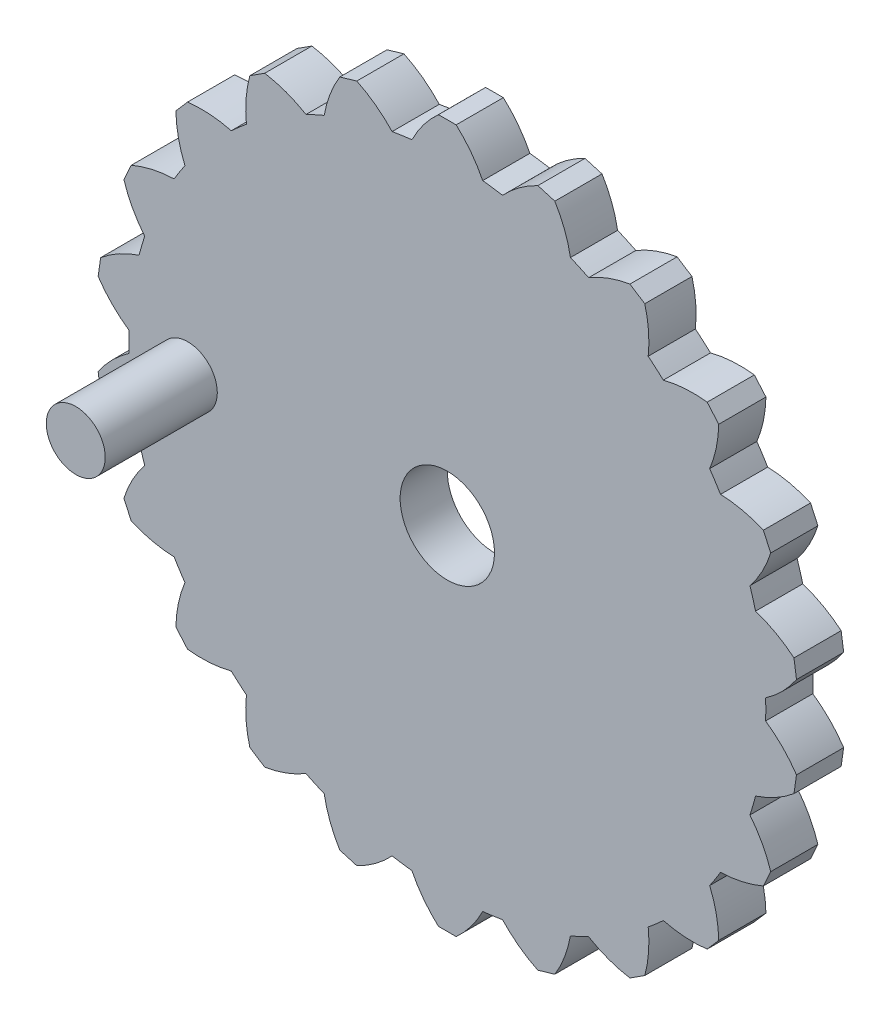
from build123d import *

# Parameters (mm, degrees)
GEAR_PROFILE_SKETCH_R = 4
GEAR_BODY_22T_DEPTH   = 4
SKETCH1_3_R           = 2.5
HUB_BOSS_DEPTH        = 9.5


with BuildPart() as part:
    # Gear Profile Sketch → Gear Body 22T (new body)
    with BuildSketch(Plane.XY):
        with BuildLine():
            Line((-0.75, 29.8), (0.75, 29.8))
            ThreePointArc((0.75, 29.8), (2.014333197, 28.422063485), (3, 26.83281573))
            ThreePointArc((3, 26.83281573), (3.842500633, 26.725178931), (4.681198862, 26.591095826))
            ThreePointArc((4.681198862, 26.591095826), (6.074682067, 27.838273451), (7.676010464, 28.804190031))
            Line((7.676010464, 28.804190031), (9.115249924, 28.381591196))
            ThreePointArc((9.115249924, 28.381591196), (9.940159165, 26.703266967), (10.438156704, 24.900700485))
            ThreePointArc((10.438156704, 24.900700485), (11.216205351, 24.560063875), (11.983154832, 24.195123481))
            ThreePointArc((11.983154832, 24.195123481), (13.671562718, 24.999192063), (15.480156211, 25.474835891))
            Line((15.480156211, 25.474835891), (16.74203651, 24.663874665))
            ThreePointArc((16.74203651, 24.663874665), (17.060692554, 22.821130571), (17.030676029, 20.951278576))
            ThreePointArc((17.030676029, 20.951278576), (17.681239817, 20.405238508), (18.314306865, 19.839006126))
            ThreePointArc((18.314306865, 19.839006126), (20.160854665, 20.13482481), (22.030191765, 20.081662052))
            Line((22.030191765, 20.081662052), (23.012482866, 18.948037691))
            ThreePointArc((23.012482866, 18.948037691), (22.799070097, 17.090161898), (22.243471269, 15.30450868))
            ThreePointArc((22.243471269, 15.30450868), (22.713845386, 14.597302071), (23.161742674, 13.875650481))
            ThreePointArc((23.161742674, 13.875650481), (25.016834069, 13.639253797), (26.795472202, 13.061591384))
            Line((26.795472202, 13.061591384), (27.418594721, 11.697143391))
            ThreePointArc((27.418594721, 11.697143391), (26.690402571, 9.974649947), (25.654232752, 8.417858509))
            ThreePointArc((25.654232752, 8.417858509), (25.906310288, 7.606779035), (26.132751841, 6.788172157))
            ThreePointArc((26.132751841, 6.788172157), (27.846098357, 6.038711558), (29.389942839, 4.983348262))
            Line((29.389942839, 4.983348262), (29.603415097, 3.498616099))
            ThreePointArc((29.603415097, 3.498616099), (28.419437363, 2.051051179), (26.98664087, 0.849243505))
            ThreePointArc((26.98664087, 0.849243505), (27, 0), (26.98664087, -0.849243505))
            ThreePointArc((26.98664087, -0.849243505), (28.419437363, -2.051051179), (29.603415097, -3.498616099))
            Line((29.603415097, -3.498616099), (29.389942839, -4.983348262))
            ThreePointArc((29.389942839, -4.983348262), (27.846098357, -6.038711558), (26.132751841, -6.788172157))
            ThreePointArc((26.132751841, -6.788172157), (25.906310288, -7.606779035), (25.654232752, -8.417858509))
            ThreePointArc((25.654232752, -8.417858509), (26.690402571, -9.974649947), (27.418594721, -11.697143391))
            Line((27.418594721, -11.697143391), (26.795472202, -13.061591384))
            ThreePointArc((26.795472202, -13.061591384), (25.016834069, -13.639253797), (23.161742674, -13.875650481))
            ThreePointArc((23.161742674, -13.875650481), (22.713845386, -14.597302071), (22.243471269, -15.30450868))
            ThreePointArc((22.243471269, -15.30450868), (22.799070097, -17.090161898), (23.012482866, -18.948037691))
            Line((23.012482866, -18.948037691), (22.030191765, -20.081662052))
            ThreePointArc((22.030191765, -20.081662052), (20.160854665, -20.13482481), (18.314306865, -19.839006126))
            ThreePointArc((18.314306865, -19.839006126), (17.681239817, -20.405238508), (17.030676029, -20.951278576))
            ThreePointArc((17.030676029, -20.951278576), (17.060692554, -22.821130571), (16.74203651, -24.663874665))
            Line((16.74203651, -24.663874665), (15.480156211, -25.474835891))
            ThreePointArc((15.480156211, -25.474835891), (13.671562718, -24.999192063), (11.983154832, -24.195123481))
            ThreePointArc((11.983154832, -24.195123481), (11.216205351, -24.560063875), (10.438156704, -24.900700485))
            ThreePointArc((10.438156704, -24.900700485), (9.940159165, -26.703266967), (9.115249924, -28.381591196))
            Line((9.115249924, -28.381591196), (7.676010464, -28.804190031))
            ThreePointArc((7.676010464, -28.804190031), (6.074682067, -27.838273451), (4.681198862, -26.591095826))
            ThreePointArc((4.681198862, -26.591095826), (3.842500633, -26.725178931), (3, -26.83281573))
            ThreePointArc((3, -26.83281573), (2.014333197, -28.422063485), (0.75, -29.8))
            Line((0.75, -29.8), (-0.75, -29.8))
            ThreePointArc((-0.75, -29.8), (-2.014333197, -28.422063485), (-3, -26.83281573))
            ThreePointArc((-3, -26.83281573), (-3.842500633, -26.725178931), (-4.681198862, -26.591095826))
            ThreePointArc((-4.681198862, -26.591095826), (-6.074682067, -27.838273451), (-7.676010464, -28.804190031))
            Line((-7.676010464, -28.804190031), (-9.115249924, -28.381591196))
            ThreePointArc((-9.115249924, -28.381591196), (-9.940159165, -26.703266967), (-10.438156704, -24.900700485))
            ThreePointArc((-10.438156704, -24.900700485), (-11.216205351, -24.560063875), (-11.983154832, -24.195123481))
            ThreePointArc((-11.983154832, -24.195123481), (-13.671562718, -24.999192063), (-15.480156211, -25.474835891))
            Line((-15.480156211, -25.474835891), (-16.74203651, -24.663874665))
            ThreePointArc((-16.74203651, -24.663874665), (-17.060692554, -22.821130571), (-17.030676029, -20.951278576))
            ThreePointArc((-17.030676029, -20.951278576), (-17.681239817, -20.405238508), (-18.314306865, -19.839006126))
            ThreePointArc((-18.314306865, -19.839006126), (-20.160854665, -20.13482481), (-22.030191765, -20.081662052))
            Line((-22.030191765, -20.081662052), (-23.012482866, -18.948037691))
            ThreePointArc((-23.012482866, -18.948037691), (-22.799070097, -17.090161898), (-22.243471269, -15.30450868))
            ThreePointArc((-22.243471269, -15.30450868), (-22.713845386, -14.597302071), (-23.161742674, -13.875650481))
            ThreePointArc((-23.161742674, -13.875650481), (-25.016834069, -13.639253797), (-26.795472202, -13.061591384))
            Line((-26.795472202, -13.061591384), (-27.418594721, -11.697143391))
            ThreePointArc((-27.418594721, -11.697143391), (-26.690402571, -9.974649947), (-25.654232752, -8.417858509))
            ThreePointArc((-25.654232752, -8.417858509), (-25.906310288, -7.606779035), (-26.132751841, -6.788172157))
            ThreePointArc((-26.132751841, -6.788172157), (-27.846098357, -6.038711558), (-29.389942839, -4.983348262))
            Line((-29.389942839, -4.983348262), (-29.603415097, -3.498616099))
            ThreePointArc((-29.603415097, -3.498616099), (-28.419437363, -2.051051179), (-26.98664087, -0.849243505))
            ThreePointArc((-26.98664087, -0.849243505), (-27, 0), (-26.98664087, 0.849243505))
            ThreePointArc((-26.98664087, 0.849243505), (-28.419437363, 2.051051179), (-29.603415097, 3.498616099))
            Line((-29.603415097, 3.498616099), (-29.389942839, 4.983348262))
            ThreePointArc((-29.389942839, 4.983348262), (-27.846098357, 6.038711558), (-26.132751841, 6.788172157))
            ThreePointArc((-26.132751841, 6.788172157), (-25.906310288, 7.606779035), (-25.654232752, 8.417858509))
            ThreePointArc((-25.654232752, 8.417858509), (-26.690402571, 9.974649947), (-27.418594721, 11.697143391))
            Line((-27.418594721, 11.697143391), (-26.795472202, 13.061591384))
            ThreePointArc((-26.795472202, 13.061591384), (-25.016834069, 13.639253797), (-23.161742674, 13.875650481))
            ThreePointArc((-23.161742674, 13.875650481), (-22.713845386, 14.597302071), (-22.243471269, 15.30450868))
            ThreePointArc((-22.243471269, 15.30450868), (-22.799070097, 17.090161898), (-23.012482866, 18.948037691))
            Line((-23.012482866, 18.948037691), (-22.030191765, 20.081662052))
            ThreePointArc((-22.030191765, 20.081662052), (-20.160854665, 20.13482481), (-18.314306865, 19.839006126))
            ThreePointArc((-18.314306865, 19.839006126), (-17.681239817, 20.405238508), (-17.030676029, 20.951278576))
            ThreePointArc((-17.030676029, 20.951278576), (-17.060692554, 22.821130571), (-16.74203651, 24.663874665))
            Line((-16.74203651, 24.663874665), (-15.480156211, 25.474835891))
            ThreePointArc((-15.480156211, 25.474835891), (-13.671562718, 24.999192063), (-11.983154832, 24.195123481))
            ThreePointArc((-11.983154832, 24.195123481), (-11.216205351, 24.560063875), (-10.438156704, 24.900700485))
            ThreePointArc((-10.438156704, 24.900700485), (-9.940159165, 26.703266967), (-9.115249924, 28.381591196))
            Line((-9.115249924, 28.381591196), (-7.676010464, 28.804190031))
            ThreePointArc((-7.676010464, 28.804190031), (-6.074682067, 27.838273451), (-4.681198862, 26.591095826))
            ThreePointArc((-4.681198862, 26.591095826), (-3.842500633, 26.725178931), (-3, 26.83281573))
            ThreePointArc((-3, 26.83281573), (-2.014333197, 28.422063485), (-0.75, 29.8))
        make_face()
        Circle(GEAR_PROFILE_SKETCH_R, mode=Mode.SUBTRACT)
    extrude(amount=-GEAR_BODY_22T_DEPTH)

    # Sketch1_3 → Hub Boss (add)
    with BuildSketch(Plane.XY):
        with Locations((-22, 0)):
            Circle(SKETCH1_3_R)
    extrude(amount=HUB_BOSS_DEPTH)


solid = part.part
